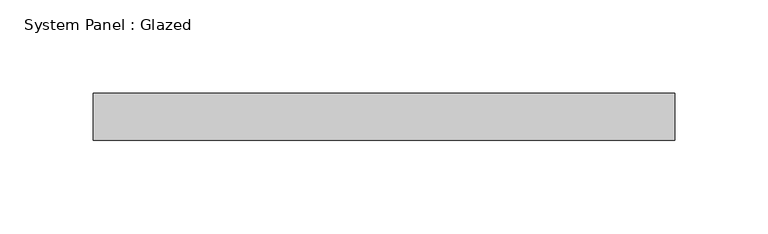
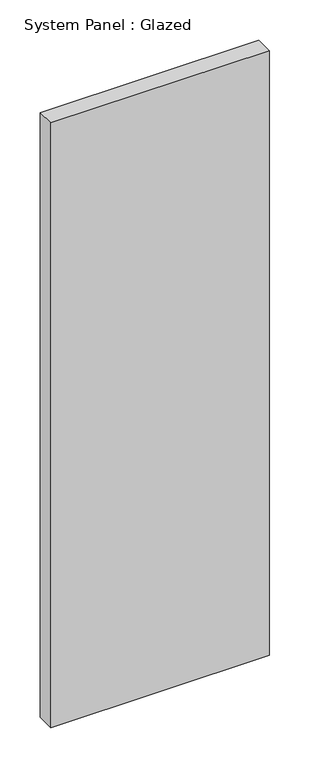
"""IFC4 building model written with IfcOpenShell, lengths in millimetres: plate geometry, System Panel : Glazed."""

from ifc_helpers import new_model, si_unit, origin, origin_with_axes, place, context, project, spatial, polyline, outline, extrude, source, transform, mapped, element, save


def system_panel_glazed_d6f392a9(model_context):
    return source(origin(), model_context, "Body", "SweptSolid", [
        extrude(outline(polyline([(156.3215916, 19.05), (-156.3215916, 19.05), (-156.3215916, 44.45), (156.3215916, 44.45), (156.3215916, 19.05)])), origin_with_axes(), (0.0, 0.0, 1.0), 914.4),
    ])


if __name__ == "__main__":
    model = new_model("IFC4")
    model_context = context("Model", 3, world=origin())
    ifc_project = project(units=[si_unit("LENGTHUNIT", "METRE", prefix="MILLI")], contexts=[model_context])
    site = spatial("IfcSite", under=ifc_project)
    building = spatial("IfcBuilding", under=site)
    placement = place(None, origin())
    system_panel_glazed_shape = system_panel_glazed_d6f392a9(model_context)
    element("IfcPlate", 1, ObjectType="System Panel : Glazed", at=placement, inside=building, context=model_context, shape_type="MappedRepresentation", body=[
        mapped(system_panel_glazed_shape, transform((0.0, 0.0, 0.0), x_axis=(1.0, 0.0, 0.0), y_axis=(0.0, 1.0, 0.0), z_axis=(0.0, 0.0, 1.0))),
    ])
    save(model, "model.ifc")

# Revit data of these elements
# Type "System Panel : Glazed"
#   Construction Type Id = "GSP4R"
#   Analytic Construction = "1/8 in Pilkington single glazing"
#   Visual Light Transmittance = 0.9
#   Solar Heat Gain Coefficient = 0.86
#   Heat Transfer Coefficient (U) = 1.18115 BTU/(h·ft²·°F)
# Element 1 (IfcPlate, "System Panel : Glazed")
#   Materials on its faces: "Glass"
# Materials
#   "Glass": class "Glass", colour RGB 0 128 192, transparency 0.75, Description = "Soda Lime Glass", Cost = 0
